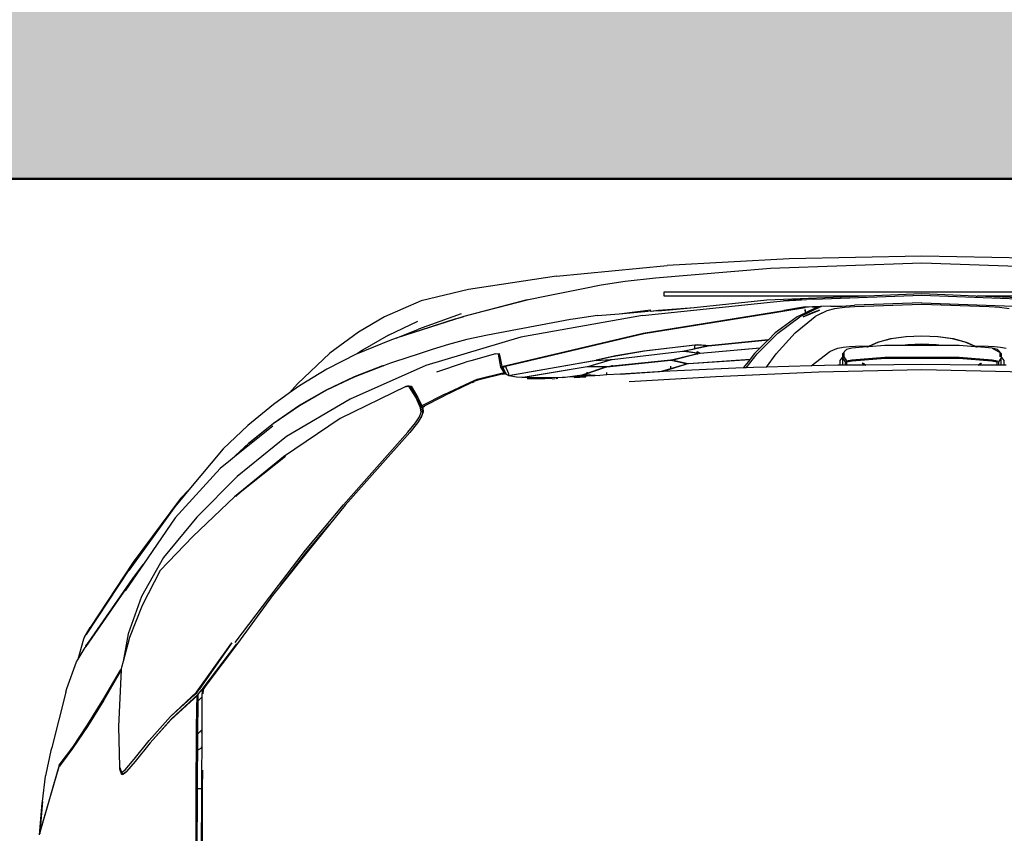
# Model space of a CAD drawing. Units: inches. Extents: x 22042254 to 25404563, y 17568978 to 17626777.
# Tile 33 of 45: x 22179810 to 22179853, y 17626366 to 17626402. Entities that reach past the tile are written whole.
import ezdxf

# ---------------------------------------------------------------- set-up
doc = ezdxf.new("R2010")
doc.units = ezdxf.units.IN
doc.header["$MEASUREMENT"] = 0
for name, color, linetype, lineweight in [('A-SITE-VEHI', 8, 'Continuous', 18), ('A-WALL-PATT', 244, 'Continuous', 13), ('walls', 252, 'Continuous', 50)]:
    doc.layers.add(name, color=color, linetype=linetype, lineweight=lineweight)
doc.layers.add('Edges', color=250, linetype='Continuous')

# ---------------------------------------------------------------- blocks, each defined once
blk = doc.blocks.new('Nissan Qashqai pl')
at = {"layer": 'Edges'}
for p, q in [((7.32157, 11.66208), (7.32157, 12.18208)), ((7.32607, 12.18208), (7.32607, 11.97794)), ((7.29801, 12.07497), (7.29279, 11.92208)), ((7.33017, 12.07853), (7.32607, 11.97794)), ((7.28835, 12.05625), (7.28572, 11.92208)), ((7.32507, 11.92208), (7.32911, 12.03155)), ((7.33294, 11.92208), (7.33653, 12.02372)), ((7.40018, 11.92208), (7.40245, 12.02601)), ((7.33733, 12.00038), (7.33865, 12.00996)), ((7.37751, 12.0015), (7.37864, 12.00699)), ((7.39094, 12.00508), (7.38696, 12.00208)), ((7.39564, 12.00508), (7.39094, 12.00508)), ((7.39588, 12.0049), (7.39564, 12.00508)), ((7.39588, 12.00508), (7.39564, 12.00508)), ((7.39588, 12.0049), (7.39584, 12.00183)), ((7.39589, 12.00706), (7.39588, 12.00508)), ((7.39588, 12.00508), (7.39588, 12.0049)), ((7.33667, 11.99003), (7.33733, 12.00038)), ((7.37648, 11.98901), (7.37683, 11.99537)), ((7.37683, 11.99537), (7.37751, 12.0015)), ((7.37985, 11.99831), (7.3787, 11.99283)), ((7.3787, 11.99283), (7.38002, 11.99534)), ((7.38081, 11.99933), (7.37985, 11.99831)), ((7.38074, 11.99908), (7.37985, 11.99831)), ((7.38002, 11.99534), (7.38305, 12.00106)), ((7.38074, 11.99908), (7.38081, 11.99933)), ((7.38104, 11.99933), (7.38074, 11.99908)), ((7.38081, 11.99933), (7.38402, 12.00208)), ((7.38104, 11.99933), (7.38081, 11.99933)), ((7.38305, 12.00106), (7.38104, 11.99933)), ((7.38659, 12.00106), (7.38305, 12.00106)), ((7.38402, 12.00208), (7.38696, 12.00208)), ((7.38683, 12.00198), (7.38659, 12.00106)), ((7.3875, 12.00106), (7.38659, 12.00106)), ((7.38696, 12.00208), (7.38683, 12.00198)), ((7.38696, 12.00208), (7.38847, 12.00208)), ((7.38847, 12.00208), (7.39254, 11.99933)), ((7.39551, 12.00208), (7.38847, 12.00208)), ((7.39041, 11.99283), (7.39156, 11.99831)), ((7.39288, 11.99808), (7.39173, 11.99259)), ((7.39254, 11.99933), (7.39582, 11.99933)), ((7.39254, 11.99933), (7.39288, 11.99808)), ((7.3958, 11.99808), (7.39288, 11.99808)), ((7.39551, 12.00208), (7.39584, 12.00183)), ((7.3958, 11.99808), (7.39564, 11.98012)), ((7.39582, 11.99933), (7.3958, 11.99808)), ((7.39584, 12.00183), (7.39582, 11.99933)), ((7.33429, 11.92208), (7.33667, 11.99003)), ((7.37614, 11.97511), (7.37648, 11.98901)), ((7.3787, 11.99283), (7.37743, 11.97775)), ((7.38759, 11.95948), (7.39041, 11.99283)), ((7.39173, 11.99259), (7.38892, 11.95935)), ((7.32607, 11.9764), (7.3238, 11.92208)), ((7.32607, 11.9764), (7.32607, 11.97794)), ((7.37239, 11.9667), (7.37614, 11.97511)), ((7.37707, 11.97569), (7.37268, 11.96585)), ((7.37727, 11.97594), (7.37588, 11.95948)), ((7.37614, 11.97511), (7.37686, 11.97673)), ((7.37686, 11.97673), (7.3771, 11.97702)), ((7.37727, 11.97594), (7.37707, 11.97569)), ((7.37713, 11.97709), (7.3771, 11.97702)), ((7.37743, 11.97775), (7.37713, 11.97709)), ((7.37713, 11.97709), (7.3774, 11.97738)), ((7.3774, 11.97738), (7.37727, 11.97594)), ((7.3774, 11.97738), (7.37743, 11.97775)), ((7.39385, 11.98229), (7.39564, 11.98012)), ((7.39563, 11.97885), (7.39385, 11.981)), ((7.39563, 11.97885), (7.3951, 11.92208)), ((7.39564, 11.98012), (7.39563, 11.97885)), ((7.36896, 11.95363), (7.37239, 11.9667)), ((7.37268, 11.96585), (7.36932, 11.95303)), ((7.37588, 11.95948), (7.37588, 11.94171)), ((7.38759, 11.88468), (7.38759, 11.95948)), ((7.38892, 11.95935), (7.38892, 11.88481)), ((7.36681, 11.93841), (7.36896, 11.95363)), ((7.36932, 11.95303), (7.3672, 11.9381)), ((7.36607, 11.92208), (7.36681, 11.93841)), ((7.3672, 11.9381), (7.36648, 11.92208)), ((7.37512, 11.93632), (7.37448, 11.92208)), ((7.37588, 11.94171), (7.37512, 11.93632)), ((7.37588, 11.94171), (7.37588, 11.93029)), ((7.37551, 11.92208), (7.37588, 11.93029)), ((7.37588, 11.93029), (7.37588, 11.91388)), ((7.28572, 11.92208), (7.28835, 11.78791)), ((7.29279, 11.92208), (7.29801, 11.76919)), ((7.3238, 11.92208), (7.32607, 11.86622)), ((7.32911, 11.81261), (7.32507, 11.92208)), ((7.33294, 11.92208), (7.33535, 11.85392)), ((7.33667, 11.85414), (7.33429, 11.92208)), ((7.36681, 11.90575), (7.36607, 11.92208)), ((7.36648, 11.92208), (7.3672, 11.90606)), ((7.37448, 11.92208), (7.37512, 11.90785)), ((7.37588, 11.91388), (7.37551, 11.92208)), ((7.3951, 11.92208), (7.39563, 11.86531)), ((7.40245, 11.81815), (7.40018, 11.92208)), ((7.36896, 11.89053), (7.36681, 11.90575)), ((7.3672, 11.90606), (7.36932, 11.89113)), ((7.37512, 11.90785), (7.37588, 11.90246)), ((7.37588, 11.91388), (7.37588, 11.90246)), ((7.37588, 11.90246), (7.37588, 11.88468)), ((7.37239, 11.87746), (7.36896, 11.89053)), ((7.36932, 11.89113), (7.37268, 11.87831)), ((7.37588, 11.88468), (7.37727, 11.86822)), ((7.39041, 11.85133), (7.38759, 11.88468)), ((7.38892, 11.88481), (7.39173, 11.85157)), ((7.37614, 11.86905), (7.37239, 11.87746)), ((7.37268, 11.87831), (7.37707, 11.86848)), ((7.32607, 11.86622), (7.33017, 11.76563)), ((7.32607, 11.86622), (7.32607, 11.66208)), ((7.37648, 11.85515), (7.37614, 11.86905)), ((7.37686, 11.86743), (7.37614, 11.86905)), ((7.3771, 11.86714), (7.37686, 11.86743)), ((7.37707, 11.86848), (7.37727, 11.86822)), ((7.3771, 11.86714), (7.37713, 11.86707)), ((7.37713, 11.86707), (7.37743, 11.86641)), ((7.3774, 11.86678), (7.37713, 11.86707)), ((7.37727, 11.86822), (7.3774, 11.86678)), ((7.3774, 11.86678), (7.37743, 11.86641)), ((7.37743, 11.86641), (7.3787, 11.85133)), ((7.39385, 11.86316), (7.39563, 11.86531)), ((7.39563, 11.86531), (7.39564, 11.86404)), ((7.37683, 11.8488), (7.37648, 11.85515)), ((7.39564, 11.86404), (7.39385, 11.86187)), ((7.39564, 11.86404), (7.3958, 11.84608)), ((7.33608, 11.84164), (7.33535, 11.85392)), ((7.33733, 11.84378), (7.33667, 11.85414)), ((7.37751, 11.84267), (7.37683, 11.8488)), ((7.3787, 11.85133), (7.37985, 11.84585)), ((7.37985, 11.84585), (7.38081, 11.84483)), ((7.38081, 11.84483), (7.38074, 11.84508)), ((7.38081, 11.84483), (7.38104, 11.84483)), ((7.38402, 11.84208), (7.38081, 11.84483)), ((7.3875, 11.8431), (7.39156, 11.84585)), ((7.39254, 11.84483), (7.38847, 11.84208)), ((7.39156, 11.84585), (7.39041, 11.85133)), ((7.39173, 11.85157), (7.39288, 11.84608)), ((7.39288, 11.84608), (7.39254, 11.84483)), ((7.39582, 11.84483), (7.39254, 11.84483)), ((7.39288, 11.84608), (7.3958, 11.84608)), ((7.3958, 11.84608), (7.39582, 11.84483)), ((7.39582, 11.84483), (7.39584, 11.84233)), ((7.33619, 11.83012), (7.33608, 11.84164)), ((7.33865, 11.8342), (7.33733, 11.84378)), ((7.37864, 11.83717), (7.37751, 11.84267)), ((7.38014, 11.8327), (7.37864, 11.83717)), ((7.38305, 11.8431), (7.3875, 11.8431)), ((7.38696, 11.84208), (7.38402, 11.84208)), ((7.38696, 11.84208), (7.39094, 11.83908)), ((7.38847, 11.84208), (7.38696, 11.84208)), ((7.39551, 11.84208), (7.38847, 11.84208)), ((7.39094, 11.83908), (7.39564, 11.83908)), ((7.39584, 11.84233), (7.39551, 11.84208)), ((7.39564, 11.83908), (7.39587, 11.83925)), ((7.39564, 11.83908), (7.39587, 11.83908)), ((7.39584, 11.84233), (7.39587, 11.83925)), ((7.39587, 11.83925), (7.39587, 11.83908)), ((7.39587, 11.83908), (7.39589, 11.8371)), ((7.39589, 11.8371), (7.3966, 11.81032)), ((7.33619, 11.83012), (7.33653, 11.82044)), ((7.3407, 11.82658), (7.33865, 11.8342)), ((7.34316, 11.82104), (7.3407, 11.82658)), ((7.38184, 11.82907), (7.38014, 11.8327)), ((7.3966, 11.81032), (7.38184, 11.82907)), ((7.33615, 11.81939), (7.33653, 11.82044)), ((7.33672, 11.81955), (7.33615, 11.81939)), ((7.33645, 11.81201), (7.33615, 11.81939)), ((7.33653, 11.82044), (7.34711, 11.79873)), ((7.33686, 11.81546), (7.33737, 11.81653)), ((7.33691, 11.81132), (7.33686, 11.81546)), ((7.33686, 11.81546), (7.33805, 11.81508)), ((7.33737, 11.81653), (7.33805, 11.81508)), ((7.33805, 11.81508), (7.34299, 11.80448)), ((7.34013, 11.81856), (7.34308, 11.8112)), ((7.347, 11.80211), (7.34013, 11.81856)), ((7.34316, 11.82104), (7.34679, 11.81424)), ((7.40723, 11.71423), (7.40245, 11.81815)), ((7.32911, 11.81261), (7.32941, 11.80569)), ((7.33008, 11.79493), (7.32941, 11.80569)), ((7.33691, 11.80472), (7.33645, 11.81201)), ((7.33691, 11.81132), (7.33767, 11.80437)), ((7.33691, 11.80472), (7.34048, 11.78254)), ((7.34308, 11.8112), (7.347, 11.80211)), ((7.36303, 11.79404), (7.34679, 11.81424)), ((7.3966, 11.81032), (7.39782, 11.76508)), ((7.3295, 11.80119), (7.33087, 11.78224)), ((7.3295, 11.80119), (7.33008, 11.79493)), ((7.33087, 11.78224), (7.33008, 11.79493)), ((7.33771, 11.80416), (7.33767, 11.80437)), ((7.34104, 11.78371), (7.33771, 11.80416)), ((7.34299, 11.80448), (7.33961, 11.8043)), ((7.33961, 11.8043), (7.34314, 11.80416)), ((7.34299, 11.80448), (7.34314, 11.80416)), ((7.34314, 11.80416), (7.34693, 11.79606)), ((7.34693, 11.79606), (7.36309, 11.77403)), ((7.36331, 11.77672), (7.34711, 11.79873)), ((7.28835, 11.78791), (7.29513, 11.66508)), ((7.38423, 11.77487), (7.36303, 11.79404)), ((7.33168, 11.77242), (7.33087, 11.78224)), ((7.36347, 11.6409), (7.34048, 11.78254)), ((7.34263, 11.77348), (7.34104, 11.78371)), ((7.38449, 11.75584), (7.36331, 11.77672)), ((7.39782, 11.76508), (7.38423, 11.77487)), ((7.29801, 11.76919), (7.30777, 11.65317)), ((7.33017, 11.76563), (7.33778, 11.69209)), ((7.34554, 11.63996), (7.33168, 11.77242)), ((7.36397, 11.64129), (7.34263, 11.77348)), ((7.36309, 11.77403), (7.37008, 11.76708)), ((7.37589, 11.71006), (7.37008, 11.76708)), ((7.37008, 11.76708), (7.37036, 11.76681)), ((7.37036, 11.76681), (7.37608, 11.71004)), ((7.37036, 11.76681), (7.37826, 11.75896)), ((7.39782, 11.76508), (7.39816, 11.75211)), ((7.38357, 11.6983), (7.37826, 11.75896)), ((7.37826, 11.75896), (7.37876, 11.75846)), ((7.37876, 11.75846), (7.38403, 11.69824)), ((7.37876, 11.75846), (7.38409, 11.75317)), ((7.39848, 11.74482), (7.38449, 11.75584)), ((7.38409, 11.75317), (7.38964, 11.74878)), ((7.39414, 11.68653), (7.38964, 11.74878)), ((7.38964, 11.74878), (7.39027, 11.74828)), ((7.39027, 11.74828), (7.39449, 11.68648)), ((7.39027, 11.74828), (7.39862, 11.74167)), ((7.39816, 11.75211), (7.39848, 11.74482)), ((7.39848, 11.74482), (7.39862, 11.74167)), ((7.39862, 11.74167), (7.40182, 11.66777)), ((7.37498, 11.69572), (7.37596, 11.70814)), ((7.37623, 11.70617), (7.37575, 11.69593)), ((7.37596, 11.70814), (7.37589, 11.71006)), ((7.37608, 11.71004), (7.37634, 11.7081)), ((7.37623, 11.70617), (7.37642, 11.70614)), ((7.37634, 11.7081), (7.38127, 11.68424)), ((7.37642, 11.70614), (7.37916, 11.6924)), ((7.41241, 11.62655), (7.40723, 11.71423)), ((7.38128, 11.64204), (7.37498, 11.69572)), ((7.37575, 11.69593), (7.37562, 11.69326)), ((7.37568, 11.69592), (7.37575, 11.69593)), ((7.38243, 11.69547), (7.38357, 11.6983)), ((7.3835, 11.69733), (7.38243, 11.69547)), ((7.38336, 11.69586), (7.38243, 11.69547)), ((7.38243, 11.69547), (7.38322, 11.69486)), ((7.38324, 11.69498), (7.38243, 11.69547)), ((7.38324, 11.69498), (7.38336, 11.69586)), ((7.3837, 11.696), (7.38336, 11.69586)), ((7.3835, 11.69733), (7.38357, 11.6983)), ((7.38361, 11.69752), (7.3835, 11.69733)), ((7.38361, 11.69752), (7.38357, 11.6983)), ((7.38403, 11.69824), (7.38361, 11.69752)), ((7.38438, 11.69629), (7.3837, 11.696)), ((7.38377, 11.69466), (7.3837, 11.696)), ((7.38426, 11.69437), (7.38438, 11.69629)), ((7.38438, 11.69629), (7.39028, 11.67251)), ((7.33778, 11.69209), (7.34072, 11.65629)), ((7.33778, 11.69209), (7.33996, 11.67104)), ((7.37916, 11.6924), (7.37562, 11.69326)), ((7.37562, 11.69326), (7.38154, 11.64126)), ((7.38118, 11.68226), (7.37916, 11.6924)), ((7.38174, 11.68442), (7.38322, 11.69486)), ((7.38379, 11.69443), (7.38202, 11.68226)), ((7.38322, 11.69486), (7.38379, 11.69443)), ((7.38377, 11.69466), (7.38324, 11.69498)), ((7.38426, 11.69437), (7.38377, 11.69466)), ((7.38429, 11.69425), (7.38379, 11.69443)), ((7.38429, 11.69425), (7.38426, 11.69437)), ((7.38773, 11.68027), (7.38429, 11.69425)), ((7.39387, 11.6846), (7.39414, 11.68653)), ((7.39449, 11.68648), (7.39509, 11.68353)), ((7.38152, 11.68035), (7.38118, 11.68226)), ((7.38127, 11.68424), (7.38174, 11.68442)), ((7.3817, 11.68412), (7.38127, 11.68424)), ((7.38995, 11.60941), (7.38152, 11.68035)), ((7.3817, 11.68412), (7.38174, 11.68442)), ((7.38202, 11.68226), (7.38195, 11.68031)), ((7.38195, 11.68031), (7.39032, 11.60945)), ((7.38737, 11.68027), (7.38773, 11.68027)), ((7.39008, 11.67074), (7.38773, 11.68027)), ((7.39093, 11.67275), (7.39387, 11.6846)), ((7.39425, 11.68274), (7.39127, 11.6705)), ((7.39425, 11.68274), (7.39494, 11.68257)), ((7.39425, 11.68274), (7.39497, 11.68247)), ((7.39497, 11.68247), (7.39494, 11.68257)), ((7.39898, 11.66858), (7.39497, 11.68247)), ((7.39509, 11.68353), (7.40207, 11.66087)), ((7.33996, 11.67104), (7.34097, 11.65941)), ((7.39046, 11.66873), (7.39008, 11.67074)), ((7.39093, 11.67275), (7.39028, 11.67251)), ((7.39087, 11.67252), (7.39028, 11.67251)), ((7.3966, 11.6095), (7.39046, 11.66873)), ((7.39087, 11.67252), (7.39093, 11.67275)), ((7.39127, 11.6705), (7.39107, 11.66865)), ((7.39107, 11.66865), (7.39768, 11.60417)), ((7.39898, 11.66858), (7.39666, 11.66858)), ((7.4017, 11.65916), (7.39898, 11.66858)), ((7.40182, 11.66777), (7.40224, 11.66093)), ((7.3059, 11.55319), (7.29513, 11.66508)), ((7.32607, 11.66208), (7.32157, 11.66208)), ((7.34072, 11.65629), (7.34131, 11.65087)), ((7.34097, 11.65941), (7.34133, 11.65108)), ((7.40216, 11.65713), (7.4017, 11.65916)), ((7.40224, 11.66093), (7.40207, 11.66087)), ((7.40224, 11.66086), (7.40207, 11.66087)), ((7.40484, 11.618), (7.40216, 11.65713)), ((7.40224, 11.66093), (7.40224, 11.66086)), ((7.40224, 11.66086), (7.40484, 11.618)), ((7.30777, 11.65317), (7.31133, 11.62243)), ((7.34009, 11.64801), (7.34004, 11.64799)), ((7.3438, 11.61665), (7.34004, 11.64799)), ((7.34097, 11.64796), (7.34009, 11.64801)), ((7.34097, 11.64796), (7.34131, 11.65087)), ((7.34097, 11.64796), (7.34145, 11.64799)), ((7.34144, 11.64796), (7.34097, 11.64796)), ((7.3438, 11.61665), (7.34121, 11.64598)), ((7.34133, 11.65108), (7.34131, 11.65087)), ((7.34131, 11.65087), (7.34154, 11.6488)), ((7.34554, 11.63996), (7.36761, 11.51724)), ((7.39705, 11.49808), (7.36347, 11.6409)), ((7.39678, 11.50175), (7.36397, 11.64129)), ((7.3869, 11.60943), (7.38128, 11.64204)), ((7.38154, 11.64126), (7.38644, 11.61311)), ((7.31133, 11.62243), (7.31494, 11.59842)), ((7.34574, 11.59466), (7.3438, 11.61665)), ((7.40484, 11.618), (7.40567, 11.60418)), ((7.38644, 11.61311), (7.39089, 11.59332)), ((7.39116, 11.59143), (7.3869, 11.60943)), ((7.39012, 11.60735), (7.38995, 11.60941)), ((7.39099, 11.59348), (7.39012, 11.60735)), ((7.39032, 11.60945), (7.3908, 11.60755)), ((7.3908, 11.60755), (7.39654, 11.58812)), ((7.3966, 11.6095), (7.39566, 11.6095)), ((7.39715, 11.60416), (7.3966, 11.6095)), ((7.31494, 11.59842), (7.3186, 11.58002)), ((7.39058, 11.60552), (7.39095, 11.60545)), ((7.39058, 11.60552), (7.39098, 11.60538)), ((7.39058, 11.60552), (7.39141, 11.59144)), ((7.39098, 11.60538), (7.39095, 11.60545)), ((7.39668, 11.58624), (7.39098, 11.60538)), ((7.39684, 11.58823), (7.39722, 11.60211)), ((7.39722, 11.60211), (7.39715, 11.60416)), ((7.39774, 11.60029), (7.39733, 11.58621)), ((7.39768, 11.60417), (7.39823, 11.60225)), ((7.39774, 11.60029), (7.39827, 11.60018)), ((7.39774, 11.60029), (7.39831, 11.60008)), ((7.39823, 11.60225), (7.40485, 11.58292)), ((7.39831, 11.60008), (7.39827, 11.60018)), ((7.40376, 11.5843), (7.39831, 11.60008)), ((7.40567, 11.60418), (7.40319, 11.60418)), ((7.40533, 11.58312), (7.40611, 11.59688)), ((7.40567, 11.60418), (7.40611, 11.59696)), ((7.40611, 11.59688), (7.40611, 11.59696)), ((7.40611, 11.59688), (7.40642, 11.59185)), ((7.34574, 11.59466), (7.34938, 11.57004)), ((7.39099, 11.59348), (7.39089, 11.59332)), ((7.39101, 11.59337), (7.39089, 11.59332)), ((7.39156, 11.58943), (7.39116, 11.59143)), ((7.39141, 11.59144), (7.39169, 11.5895)), ((7.40622, 11.5053), (7.39156, 11.58943)), ((7.39169, 11.5895), (7.40648, 11.50498)), ((7.39684, 11.58823), (7.39654, 11.58812)), ((7.39714, 11.58424), (7.39668, 11.58624)), ((7.39684, 11.58823), (7.39731, 11.58844)), ((7.39733, 11.58621), (7.39747, 11.58427)), ((7.40642, 11.59185), (7.40597, 11.58338)), ((7.40642, 11.59185), (7.40687, 11.58436)), ((7.3186, 11.58002), (7.32232, 11.56164)), ((7.40828, 11.51835), (7.39714, 11.58424)), ((7.39747, 11.58427), (7.40836, 11.51976)), ((7.40376, 11.5843), (7.40279, 11.5843)), ((7.40488, 11.58107), (7.40376, 11.5843)), ((7.40533, 11.58312), (7.40485, 11.58292)), ((7.40532, 11.58299), (7.40485, 11.58292)), ((7.40539, 11.57906), (7.40488, 11.58107)), ((7.40597, 11.58327), (7.40532, 11.58299)), ((7.40532, 11.58299), (7.40533, 11.58312)), ((7.40597, 11.58338), (7.40533, 11.58312)), ((7.40814, 11.55935), (7.40539, 11.57906)), ((7.40597, 11.58327), (7.40585, 11.58097)), ((7.40585, 11.58097), (7.40588, 11.57905)), ((7.40588, 11.57905), (7.40791, 11.56437)), ((7.40597, 11.58338), (7.40597, 11.58327)), ((7.40687, 11.58436), (7.40791, 11.56437)), ((7.40813, 11.57111), (7.40752, 11.58276)), ((7.34938, 11.57004), (7.3497, 11.56742)), ((7.34938, 11.57004), (7.34978, 11.56736)), ((7.3497, 11.56742), (7.36534, 11.48377)), ((7.32232, 11.56164), (7.3261, 11.54328)), ((7.40791, 11.56437), (7.40811, 11.56038)), ((7.40791, 11.56437), (7.40812, 11.56285)), ((7.40811, 11.56038), (7.40814, 11.55935)), ((7.40814, 11.55935), (7.40871, 11.54047)), ((7.3059, 11.55319), (7.31925, 11.46451)), ((7.40923, 11.54161), (7.40902, 11.54853)), ((7.4096, 11.54898), (7.40916, 11.55209)), ((7.40926, 11.55458), (7.40949, 11.55292)), ((7.3261, 11.54328), (7.32996, 11.52493)), ((7.40871, 11.54047), (7.40865, 11.52464)), ((7.40921, 11.52579), (7.40923, 11.54161)), ((7.3297, 11.52373), (7.34671, 11.45961)), ((7.32996, 11.52493), (7.34671, 11.45961)), ((7.36761, 11.51724), (7.39627, 11.42146)), ((7.40828, 11.51835), (7.40795, 11.51289)), ((7.40836, 11.51976), (7.40828, 11.51835)), ((7.40865, 11.52464), (7.40836, 11.51976)), ((7.40908, 11.52353), (7.40921, 11.52579)), ((7.40795, 11.51289), (7.4066, 11.50521)), ((7.39764, 11.49714), (7.38458, 11.49463)), ((7.38529, 11.49584), (7.39705, 11.49808)), ((7.40464, 11.5053), (7.39678, 11.50175)), ((7.39804, 11.49925), (7.39678, 11.50175)), ((7.39705, 11.49808), (7.39833, 11.49833)), ((7.40264, 11.50022), (7.39764, 11.49714)), ((7.39804, 11.49925), (7.40478, 11.50242)), ((7.4012, 11.50009), (7.39804, 11.49925)), ((7.39833, 11.49833), (7.4012, 11.50009)), ((7.4012, 11.50009), (7.40335, 11.50141)), ((7.40299, 11.50047), (7.40264, 11.50022)), ((7.40299, 11.50047), (7.40276, 11.50042)), ((7.40326, 11.50066), (7.40299, 11.50047)), ((7.40417, 11.50199), (7.40326, 11.50066)), ((7.4033, 11.50053), (7.40326, 11.50066)), ((7.40335, 11.50054), (7.4033, 11.50053)), ((7.41007, 11.47333), (7.4033, 11.50053)), ((7.40335, 11.50141), (7.40417, 11.50199)), ((7.40425, 11.50164), (7.40405, 11.50122)), ((7.40431, 11.5014), (7.40405, 11.50122)), ((7.40405, 11.50122), (7.41077, 11.47382)), ((7.40417, 11.50199), (7.40443, 11.50199)), ((7.40425, 11.50164), (7.40417, 11.50199)), ((7.40443, 11.50199), (7.40425, 11.50164)), ((7.40431, 11.5014), (7.40425, 11.50164)), ((7.40461, 11.50161), (7.40431, 11.5014)), ((7.40447, 11.50076), (7.40431, 11.5014)), ((7.40456, 11.50227), (7.40443, 11.50199)), ((7.40443, 11.50199), (7.40463, 11.50199)), ((7.4048, 11.50082), (7.40447, 11.50076)), ((7.40502, 11.49854), (7.40447, 11.50076)), ((7.40456, 11.50227), (7.40478, 11.50242)), ((7.40497, 11.50227), (7.40456, 11.50227)), ((7.40456, 11.50227), (7.40463, 11.50199)), ((7.40469, 11.50176), (7.40461, 11.50161)), ((7.40463, 11.50199), (7.40469, 11.50176)), ((7.40463, 11.50199), (7.40482, 11.50199)), ((7.40622, 11.5053), (7.40464, 11.5053)), ((7.40482, 11.50199), (7.40469, 11.50176)), ((7.40478, 11.50242), (7.40523, 11.50274)), ((7.40515, 11.5026), (7.40478, 11.50242)), ((7.40497, 11.50227), (7.40482, 11.50199)), ((7.40515, 11.5026), (7.40497, 11.50227)), ((7.40523, 11.50274), (7.40515, 11.5026)), ((7.40632, 11.5047), (7.40523, 11.50274)), ((7.40632, 11.5047), (7.40622, 11.5053)), ((7.40648, 11.50498), (7.40632, 11.5047)), ((7.4066, 11.50521), (7.40648, 11.50498)), ((7.38529, 11.49584), (7.38412, 11.49562)), ((7.38437, 11.49158), (7.38412, 11.49562)), ((7.38458, 11.49463), (7.38437, 11.49158)), ((7.38437, 11.49158), (7.39136, 11.46669)), ((7.38529, 11.49584), (7.38458, 11.49463)), ((7.36534, 11.48377), (7.36995, 11.46286)), ((7.41147, 11.46951), (7.41007, 11.47333)), ((7.41077, 11.47382), (7.41219, 11.47)), ((7.41315, 11.46587), (7.41147, 11.46951)), ((7.41219, 11.47), (7.41393, 11.46637)), ((7.41256, 11.46999), (7.41248, 11.47021)), ((7.41324, 11.46853), (7.41256, 11.46999)), ((7.31925, 11.46451), (7.3309, 11.41659)), ((7.34401, 11.45722), (7.35959, 11.41392)), ((7.34891, 11.45171), (7.34671, 11.45961)), ((7.34671, 11.45961), (7.36864, 11.39135)), ((7.36995, 11.46286), (7.375, 11.44419)), ((7.39136, 11.46669), (7.39248, 11.46286)), ((7.39248, 11.46286), (7.39374, 11.45905)), ((7.39374, 11.45905), (7.40289, 11.43211)), ((7.42553, 11.43981), (7.41315, 11.46587)), ((7.41393, 11.46637), (7.42672, 11.44006)), ((7.34891, 11.45171), (7.36864, 11.39135)), ((7.375, 11.44419), (7.37986, 11.42777)), ((7.42553, 11.43981), (7.43673, 11.41738)), ((7.43787, 11.41791), (7.42672, 11.44006)), ((7.37986, 11.42777), (7.38454, 11.41358)), ((7.39627, 11.42146), (7.43015, 11.3449)), ((7.43587, 11.41698), (7.43673, 11.41738)), ((7.43832, 11.417), (7.43673, 11.41738)), ((7.43751, 11.42004), (7.43844, 11.41817)), ((7.43787, 11.41791), (7.43844, 11.41817)), ((7.4389, 11.41727), (7.43787, 11.41791)), ((7.43832, 11.417), (7.43787, 11.41791)), ((7.4389, 11.41727), (7.43832, 11.417)), ((7.43844, 11.41817), (7.43873, 11.41831)), ((7.43873, 11.41831), (7.44298, 11.41881)), ((7.4389, 11.41727), (7.44004, 11.41781)), ((7.44418, 11.41831), (7.44004, 11.41781)), ((7.44298, 11.41881), (7.44771, 11.41717)), ((7.44771, 11.41717), (7.44418, 11.41831)), ((7.44771, 11.41717), (7.45415, 11.41285)), ((7.3309, 11.41659), (7.34698, 11.37976)), ((7.36552, 11.38372), (7.3514, 11.41334)), ((7.36864, 11.39135), (7.35959, 11.41392)), ((7.38454, 11.41358), (7.39247, 11.38995)), ((7.42821, 11.41133), (7.41689, 11.40438)), ((7.41697, 11.40649), (7.42833, 11.41346)), ((7.42961, 11.41292), (7.4183, 11.40596)), ((7.43873, 11.41619), (7.42821, 11.41133)), ((7.42833, 11.41346), (7.43587, 11.41698)), ((7.42961, 11.41292), (7.43832, 11.417)), ((7.44309, 11.41655), (7.43873, 11.41619)), ((7.44789, 11.41487), (7.44309, 11.41655)), ((7.4541, 11.41081), (7.44789, 11.41487)), ((7.46355, 11.40337), (7.4541, 11.41081)), ((7.45415, 11.41285), (7.46382, 11.40513)), ((7.41665, 11.40488), (7.41697, 11.40649)), ((7.41716, 11.40469), (7.41665, 11.40488)), ((7.41687, 11.40359), (7.41665, 11.40488)), ((7.41687, 11.40359), (7.41686, 11.40296)), ((7.41686, 11.40296), (7.41723, 11.40107)), ((7.41689, 11.40438), (7.41687, 11.40359)), ((7.41717, 11.40184), (7.41687, 11.40359)), ((7.41716, 11.40469), (7.41689, 11.40438)), ((7.4183, 11.40596), (7.41716, 11.40469)), ((7.41744, 11.4013), (7.41717, 11.40184)), ((7.41723, 11.40107), (7.44978, 11.33488)), ((7.41744, 11.4013), (7.41747, 11.40124)), ((7.53689, 11.33848), (7.46355, 11.40337)), ((7.46382, 11.40513), (7.53708, 11.33997)), ((7.36864, 11.39135), (7.37074, 11.38491)), ((7.39247, 11.38995), (7.39379, 11.3859)), ((7.34698, 11.37976), (7.36237, 11.35349)), ((7.36552, 11.38372), (7.38053, 11.35758)), ((7.37074, 11.38491), (7.38426, 11.35219)), ((7.39379, 11.3859), (7.39513, 11.38217)), ((7.39513, 11.38217), (7.39648, 11.37869)), ((7.39621, 11.37814), (7.39648, 11.37869)), ((7.40715, 11.34933), (7.39621, 11.37814)), ((7.39648, 11.37869), (7.39687, 11.3777)), ((7.39687, 11.3777), (7.40781, 11.34902)), ((7.38053, 11.35758), (7.38426, 11.35219)), ((7.36237, 11.35349), (7.38367, 11.32447)), ((7.38426, 11.35219), (7.38446, 11.35171)), ((7.38446, 11.35171), (7.39973, 11.32146)), ((7.42053, 11.32124), (7.40715, 11.34933)), ((7.40781, 11.34902), (7.42115, 11.32101)), ((7.43015, 11.3449), (7.46788, 11.28072)), ((7.58274, 11.30006), (7.53689, 11.33848)), ((7.53708, 11.33997), (7.55684, 11.32404)), ((7.44978, 11.33488), (7.48836, 11.27781)), ((7.38367, 11.32447), (7.41469, 11.29179)), ((7.39973, 11.32146), (7.41661, 11.29389)), ((7.43626, 11.29398), (7.42053, 11.32124)), ((7.42115, 11.32101), (7.4369, 11.29377)), ((7.58398, 11.30127), (7.55684, 11.32404)), ((7.55684, 11.32404), (7.58288, 11.30303)), ((7.6296, 11.2639), (7.58274, 11.30006)), ((7.58288, 11.30303), (7.61803, 11.27504)), ((7.61803, 11.27504), (7.58398, 11.30127)), ((7.41469, 11.29179), (7.42386, 11.28371)), ((7.41661, 11.29389), (7.42386, 11.28371)), ((7.45423, 11.26769), (7.43626, 11.29398)), ((7.4369, 11.29377), (7.45491, 11.26748)), ((7.42386, 11.28371), (7.4354, 11.26752)), ((7.46788, 11.28072), (7.50805, 11.2311)), ((7.48817, 11.27966), (7.52431, 11.23409)), ((7.48836, 11.27781), (7.52891, 11.22832)), ((7.61803, 11.27504), (7.63007, 11.26544)), ((7.4354, 11.26752), (7.45654, 11.24186)), ((7.47438, 11.24268), (7.45423, 11.26769)), ((7.45491, 11.26748), (7.47504, 11.24255)), ((7.45735, 11.26699), (7.48846, 11.22834)), ((7.67598, 11.22893), (7.6296, 11.2639)), ((7.63007, 11.26544), (7.63056, 11.26506)), ((7.63056, 11.26506), (7.63059, 11.26504)), ((7.63059, 11.26504), (7.6373, 11.26013)), ((7.6373, 11.26013), (7.67691, 11.23122)), ((7.45654, 11.24186), (7.48015, 11.2168)), ((7.49177, 11.22424), (7.47438, 11.24268)), ((7.47504, 11.24255), (7.47703, 11.24044)), ((7.47703, 11.24044), (7.47653, 11.24106)), ((7.47703, 11.24053), (7.47751, 11.23993)), ((7.47838, 11.23878), (7.47703, 11.24044)), ((7.47703, 11.24044), (7.47751, 11.23993)), ((7.47751, 11.23993), (7.47871, 11.23847)), ((7.47751, 11.23993), (7.47869, 11.23868)), ((7.47869, 11.23868), (7.47824, 11.23925)), ((7.4795, 11.2377), (7.47869, 11.23868)), ((7.47869, 11.23868), (7.48846, 11.22834)), ((7.48846, 11.22834), (7.49177, 11.22424)), ((7.50805, 11.2311), (7.5492, 11.19016)), ((7.52431, 11.23409), (7.52857, 11.22958)), ((7.52891, 11.22832), (7.56866, 11.18624)), ((7.67691, 11.23122), (7.71943, 11.19922)), ((7.72318, 11.19554), (7.67713, 11.2307)), ((7.49177, 11.22424), (7.50008, 11.21391)), ((7.72614, 11.18985), (7.67617, 11.22557)), ((7.67617, 11.22557), (7.72327, 11.1928)), ((7.48015, 11.2168), (7.52174, 11.18228)), ((7.50008, 11.21391), (7.55011, 11.16843)), ((7.71943, 11.19922), (7.72318, 11.19658)), ((7.5492, 11.19016), (7.58999, 11.1565)), ((7.72318, 11.19658), (7.72785, 11.19647)), ((7.72807, 11.19181), (7.72318, 11.19554)), ((7.72318, 11.19554), (7.72455, 11.19553)), ((7.72667, 11.19023), (7.72327, 11.1928)), ((7.72467, 11.19542), (7.72455, 11.19553)), ((7.72455, 11.19553), (7.72942, 11.19548)), ((7.72614, 11.18985), (7.75074, 11.16383)), ((7.72856, 11.18809), (7.72667, 11.19023)), ((7.72807, 11.19181), (7.72986, 11.19044)), ((7.73491, 11.19175), (7.72807, 11.19181)), ((7.75301, 11.16475), (7.72807, 11.19181)), ((7.72942, 11.19548), (7.73096, 11.19549)), ((7.72986, 11.19044), (7.73238, 11.18764)), ((7.72986, 11.19044), (7.73635, 11.19039)), ((7.73096, 11.19549), (7.73491, 11.19175)), ((7.73096, 11.19549), (7.76399, 11.19528)), ((7.76799, 11.19147), (7.73491, 11.19175)), ((7.7363, 11.19044), (7.73635, 11.19039)), ((7.76942, 11.19011), (7.73635, 11.19039)), ((7.76399, 11.19528), (7.7636, 11.19566)), ((7.76799, 11.19147), (7.76399, 11.19528)), ((7.76399, 11.19528), (7.76622, 11.19527)), ((7.76586, 11.19567), (7.76622, 11.19527)), ((7.76622, 11.19527), (7.76683, 11.19458)), ((7.76622, 11.19527), (7.78115, 11.19519)), ((7.76925, 11.19146), (7.76799, 11.19147)), ((7.76942, 11.19011), (7.76874, 11.19075)), ((7.78439, 11.19133), (7.76925, 11.19146)), ((7.7707, 11.1901), (7.76942, 11.19011)), ((7.78514, 11.18998), (7.7707, 11.1901)), ((7.78115, 11.19519), (7.78091, 11.19575)), ((7.7814, 11.19458), (7.78115, 11.19519)), ((7.78115, 11.19519), (7.78224, 11.19518)), ((7.78224, 11.19518), (7.78192, 11.19576)), ((7.78224, 11.19518), (7.80566, 11.19505)), ((7.78439, 11.19133), (7.78224, 11.19518)), ((7.80777, 11.19113), (7.78439, 11.19133)), ((7.78462, 11.19091), (7.78514, 11.18998)), ((7.80829, 11.18979), (7.78514, 11.18998)), ((7.80482, 11.19588), (7.82329, 11.1958)), ((7.80566, 11.19505), (7.82329, 11.19498)), ((7.82329, 11.19107), (7.80777, 11.19113)), ((7.90396, 11.18944), (7.80829, 11.18979)), ((7.82329, 11.19498), (7.82329, 11.1958)), ((7.82329, 11.1958), (7.90142, 11.19549)), ((7.82329, 11.19498), (7.90204, 11.19468)), ((7.82329, 11.19107), (7.82329, 11.19498)), ((7.82329, 11.18994), (7.82329, 11.19107)), ((7.90357, 11.19074), (7.82329, 11.19107)), ((7.53043, 11.17373), (7.52174, 11.18228)), ((7.52174, 11.18228), (7.53868, 11.16822)), ((7.56866, 11.18624), (7.60319, 11.15334)), ((7.75074, 11.16383), (7.72856, 11.18809)), ((7.73238, 11.18764), (7.75388, 11.16419)), ((7.53043, 11.17373), (7.59458, 11.12619)), ((7.53868, 11.16822), (7.60312, 11.12171)), ((7.55011, 11.16843), (7.59689, 11.13645)), ((7.77477, 11.14231), (7.75074, 11.16383)), ((7.75301, 11.16475), (7.77724, 11.14311)), ((7.75388, 11.16419), (7.77724, 11.14311)), ((7.58999, 11.1565), (7.62951, 11.13442)), ((7.60319, 11.15334), (7.63858, 11.13525)), ((7.79381, 11.1271), (7.77477, 11.14231)), ((7.77724, 11.14311), (7.79586, 11.12808)), ((7.61132, 11.12557), (7.59689, 11.13645)), ((7.59689, 11.13645), (7.6021, 11.13289)), ((7.6021, 11.13289), (7.61183, 11.12554)), ((7.6021, 11.13289), (7.62368, 11.11814)), ((7.62951, 11.13442), (7.66697, 11.12116)), ((7.63858, 11.13525), (7.67084, 11.12249)), ((7.59458, 11.12619), (7.66077, 11.0825)), ((7.66763, 11.07907), (7.60245, 11.12206)), ((7.67585, 11.08087), (7.61132, 11.12557)), ((7.61183, 11.12554), (7.67993, 11.07831)), ((7.66697, 11.12116), (7.69488, 11.11584)), ((7.67084, 11.12249), (7.69488, 11.11584)), ((7.80447, 11.11791), (7.79381, 11.1271)), ((7.79586, 11.12808), (7.80619, 11.11916)), ((7.80867, 11.11585), (7.80619, 11.11916)), ((7.80619, 11.11916), (7.80665, 11.11877)), ((7.69488, 11.11584), (7.70101, 11.11415)), ((7.70101, 11.11415), (7.70235, 11.11408)), ((7.70382, 11.11316), (7.70235, 11.11408)), ((7.70235, 11.11408), (7.70343, 11.11403)), ((7.70343, 11.11403), (7.70559, 11.11279)), ((7.70343, 11.11403), (7.76082, 11.11124)), ((7.73247, 11.09659), (7.70382, 11.11316)), ((7.70559, 11.11279), (7.73411, 11.09632)), ((7.76082, 11.11124), (7.80143, 11.11238)), ((7.80143, 11.11238), (7.80216, 11.1126)), ((7.80216, 11.1126), (7.80721, 11.11412)), ((7.80372, 11.11265), (7.80216, 11.1126)), ((7.80956, 11.11476), (7.80372, 11.11265)), ((7.80721, 11.11412), (7.80447, 11.11791)), ((7.80665, 11.11877), (7.80956, 11.11476)), ((7.80721, 11.11412), (7.80867, 11.11585)), ((7.75906, 11.08002), (7.73247, 11.09659)), ((7.73411, 11.09632), (7.76061, 11.0798)), ((7.67122, 11.0767), (7.66077, 11.0825)), ((7.67933, 11.07844), (7.67585, 11.08087)), ((7.78138, 11.06503), (7.75906, 11.08002)), ((7.76061, 11.0798), (7.78285, 11.06486)), ((7.67207, 11.07622), (7.67122, 11.0767)), ((7.6926, 11.07047), (7.67207, 11.07622)), ((7.68018, 11.07816), (7.67933, 11.07844)), ((7.68018, 11.07816), (7.67993, 11.07831)), ((7.68089, 11.07772), (7.68018, 11.07816)), ((7.6926, 11.07047), (7.68089, 11.07772)), ((7.69527, 11.06881), (7.6926, 11.07047)), ((7.72226, 11.05905), (7.69527, 11.06881)), ((7.79699, 11.05342), (7.78138, 11.06503)), ((7.78285, 11.06486), (7.79842, 11.05331)), ((7.72615, 11.0581), (7.72226, 11.05905)), ((7.72615, 11.0581), (7.78191, 11.04384)), ((7.79699, 11.05342), (7.79703, 11.05339)), ((7.79979, 11.05134), (7.79703, 11.05339)), ((7.79842, 11.05331), (7.80074, 11.05158)), ((7.79979, 11.05134), (7.86763, 11.03183)), ((7.80074, 11.05158), (7.80015, 11.05168)), ((7.80074, 11.05158), (7.80119, 11.05125)), ((7.86805, 11.03202), (7.80119, 11.05125)), ((7.78191, 11.04384), (7.78484, 11.043)), ((7.78484, 11.043), (7.80866, 11.03796)), ((7.80866, 11.03796), (7.81062, 11.03771)), ((7.81073, 11.03768), (7.81062, 11.03771)), ((7.83626, 11.03444), (7.81073, 11.03768)), ((7.83812, 11.0342), (7.83626, 11.03444)), ((7.83626, 11.03444), (7.86763, 11.03183)), ((7.86997, 11.03154), (7.83812, 11.0342)), ((7.86805, 11.03202), (7.86763, 11.03183)), ((7.86805, 11.03202), (7.86903, 11.03174))]:
    blk.add_line(p, q, dxfattribs=at)
blk = doc.blocks.new('CAR')
blk.add_blockref('Nissan Qashqai pl', (-9.74328, -11.91512))

msp = doc.modelspace()

# ---------------------------------------------------------------- hatches: boundary and pattern name
at = {"layer": 'A-WALL-PATT'}
h = msp.add_hatch(color=256, dxfattribs=at)
h.dxf.hatch_style = 1
h.paths.add_polyline_path([(22179792.734, 17626580.28), (22179888.734, 17626580.28), (22179888.734, 17626559.623), (22179893.234, 17626559.623), (22179893.234, 17626580.28), (22179900.438, 17626580.28), (22179900.438, 17626584.78), (22179792.734, 17626584.78), (22179792.734, 17626728.78), (22180134.734, 17626728.78), (22180134.734, 17626584.78), (22180035.602, 17626584.78), (22180004.432, 17626584.78), (22180001.734, 17626584.78), (22180001.734, 17626580.28), (22180134.734, 17626580.28), (22180134.734, 17626404.28), (22180064.487, 17626404.28), (22180064.487, 17626399.78), (22180134.734, 17626399.78), (22180134.734, 17626197.78), (22180143.734, 17626197.78), (22180143.734, 17626737.78), (22179783.734, 17626737.78), (22179783.734, 17626197.78), (22179792.734, 17626197.78), (22179792.734, 17626394.78), (22179936.734, 17626394.78), (22179936.734, 17626383.208), (22179941.234, 17626383.208), (22179941.234, 17626532.28), (22179927.066, 17626532.28), (22179927.066, 17626527.78), (22179928.072, 17626527.78), (22179936.734, 17626527.78), (22179936.734, 17626403.78), (22179792.734, 17626403.78), (22179792.734, 17626527.78), (22179905.094, 17626527.78), (22179905.094, 17626532.28), (22179792.734, 17626532.28)])

# ---------------------------------------------------------------- linework, layer by layer
at = {"layer": 'walls'}
msp.add_line((22179792.734, 17626394.78), (22179936.734, 17626394.78), dxfattribs=at)

# ---------------------------------------------------------------- block references
at = {"layer": 'A-SITE-VEHI', "xscale": 43.56002006885659, "yscale": 43.56002006885659, "zscale": 43.56002006885659, "rotation": 270}
msp.add_blockref('CAR', (22179848.861, 17626284.325), dxfattribs=at)

doc.saveas('drawing.dxf')
